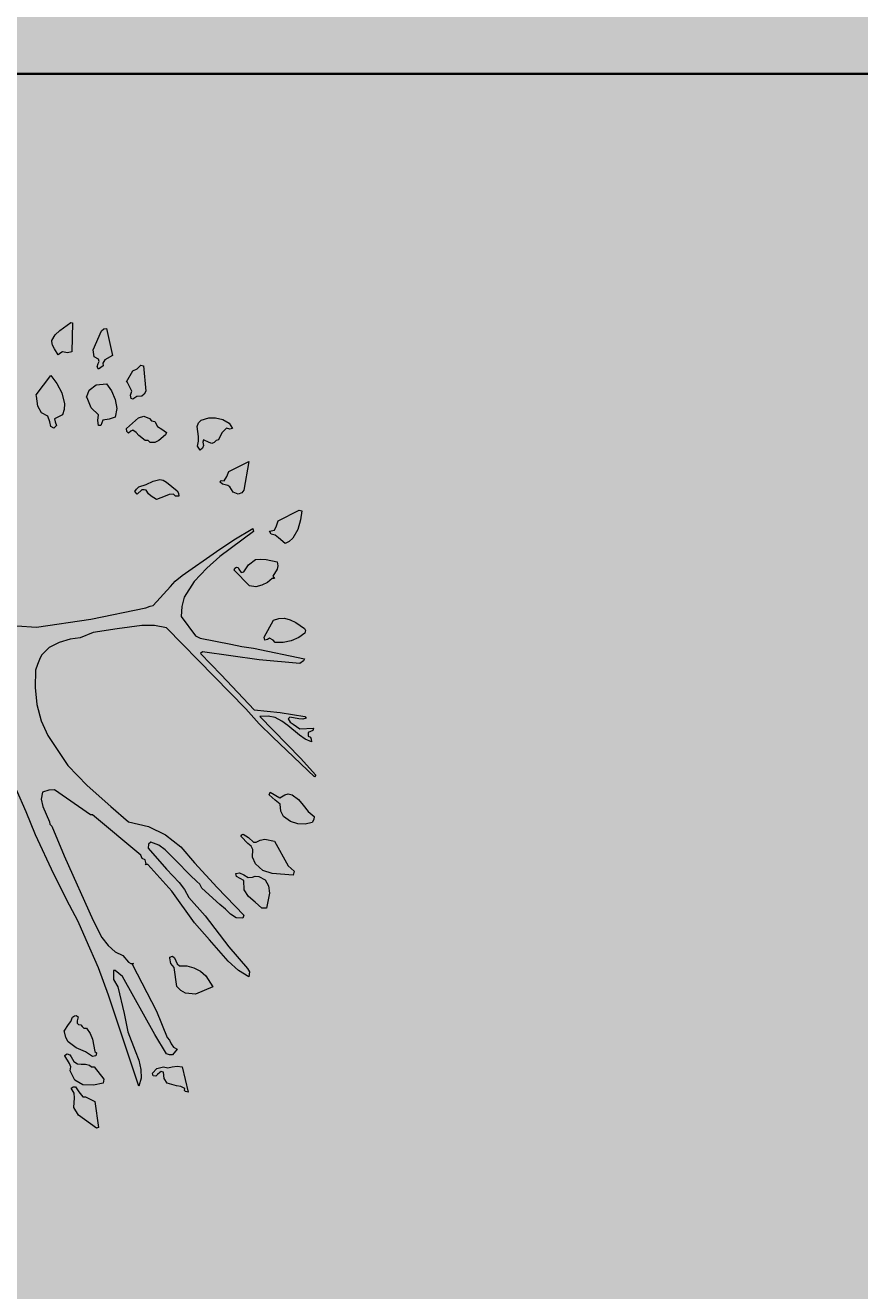
# Model space of a CAD drawing. Units: inches. Extents: x 84 to 1044, y -280 to 906.
# Tile 96 of 105: x 804 to 826, y 479 to 512. Entities that reach past the tile are written whole.
import ezdxf

# ---------------------------------------------------------------- set-up
doc = ezdxf.new("R2010")
doc.units = ezdxf.units.IN
for name, color, linetype, lineweight in [('A-ANNO-DIMS', 2, 'Continuous', 18), ('L-PLNT', 114, 'Continuous', 15), ('WALL', 250, 'Continuous', 35)]:
    doc.layers.add(name, color=color, linetype=linetype, lineweight=lineweight)
doc.layers.add('A-WALL-PATT', color=251, linetype='Continuous', lineweight=9, true_color=0x636466)
doc.layers.add('L-PLNT-PATT', color=9, linetype='Continuous', lineweight=9, true_color=0xafd9aa)
doc.styles.get("Standard").update_dxf_attribs({"font": 'arial.ttf'})
doc.dimstyles.get("Standard").update_dxf_attribs({"dimtxt": 0.18, "dimasz": 0.18, "dimexe": 0.18, "dimexo": 0.0625, "dimgap": 0.09, "dimtad": 0, "dimtih": 1, "dimtoh": 1, "dimdec": 4, "dimzin": 0, "dimdsep": 46, "dimtxsty": 'Standard', "dimcen": 0.09, "dimadec": 0, "dimazin": 0, "dimtfac": 1, "dimtdec": 4, "dimtofl": 0, "dimtmove": 0, "dimatfit": 3, "dimfxl": 1, "dimtolj": 1, "dimtzin": 0, "dimarcsym": 0})

# ---------------------------------------------------------------- blocks, each defined once
blk = doc.blocks.new('A$C37E508DF')
for p, q in [((0.9605, 1.4257), (0.9686, 1.4334)), ((0.9686, 1.4334), (0.9875, 1.4476)), ((0.9875, 1.4476), (0.9905, 1.4467)), ((0.9905, 1.4467), (0.9896, 1.3966)), ((1.0269, 1.3996), (1.0411, 1.433)), ((1.0411, 1.433), (1.045, 1.4365)), ((1.045, 1.4365), (1.0497, 1.4369)), ((1.0497, 1.4369), (1.0604, 1.3901)), ((0.9545, 1.4159), (0.9605, 1.4257)), ((0.9549, 1.4146), (0.9545, 1.4159)), ((0.9558, 1.4077), (0.9549, 1.4146)), ((0.9592, 1.4017), (0.9558, 1.4077)), ((0.966, 1.3914), (0.9592, 1.4017)), ((0.9703, 1.3944), (0.966, 1.3914)), ((0.9733, 1.3966), (0.9703, 1.3944)), ((0.9819, 1.3944), (0.9733, 1.3966)), ((0.9896, 1.3966), (0.9819, 1.3944)), ((1.0282, 1.3876), (1.0269, 1.3996)), ((1.0359, 1.3833), (1.0282, 1.3876)), ((1.0604, 1.3901), (1.0471, 1.3824)), ((1.0334, 1.37), (1.0351, 1.376)), ((1.0359, 1.3661), (1.0334, 1.37)), ((1.0351, 1.376), (1.0368, 1.3794)), ((1.0368, 1.3794), (1.0359, 1.3833)), ((1.0441, 1.3717), (1.0359, 1.3661)), ((1.0471, 1.3824), (1.0432, 1.3764)), ((1.0432, 1.3764), (1.0441, 1.3717)), ((1.0955, 1.3631), (1.1033, 1.367)), ((1.1033, 1.367), (1.1097, 1.373)), ((1.1097, 1.373), (1.114, 1.3717)), ((1.114, 1.3717), (1.1183, 1.328)), ((0.9274, 1.3215), (0.9532, 1.3554)), ((0.9532, 1.3554), (0.9635, 1.3413)), ((1.0848, 1.3443), (1.0955, 1.3631)), ((1.0861, 1.343), (1.0848, 1.3443)), ((0.9279, 1.3194), (0.9274, 1.3215)), ((0.9635, 1.3413), (0.9721, 1.325)), ((0.9721, 1.325), (0.9768, 1.3061)), ((1.0149, 1.3172), (1.0171, 1.3232)), ((1.0171, 1.3232), (1.0197, 1.3297)), ((1.0197, 1.3297), (1.0321, 1.3387)), ((1.0321, 1.3387), (1.0497, 1.3404)), ((1.0497, 1.3404), (1.0587, 1.3284)), ((1.0587, 1.3284), (1.0651, 1.3134)), ((1.0938, 1.328), (1.0861, 1.343)), ((1.0917, 1.3207), (1.0938, 1.328)), ((1.1153, 1.3228), (1.111, 1.3194)), ((1.1183, 1.328), (1.1153, 1.3228)), ((0.9305, 1.3018), (0.9279, 1.3194)), ((0.9365, 1.2902), (0.9305, 1.3018)), ((0.9768, 1.3061), (0.9763, 1.2962)), ((1.0162, 1.3164), (1.0149, 1.3172)), ((1.0231, 1.2988), (1.0162, 1.3164)), ((1.0651, 1.3134), (1.0677, 1.2975)), ((1.0925, 1.3151), (1.0917, 1.3207)), ((1.0955, 1.3138), (1.0925, 1.3151)), ((1.1028, 1.3185), (1.0955, 1.3138)), ((1.111, 1.3194), (1.1028, 1.3185)), ((0.9476, 1.2842), (0.9365, 1.2902)), ((0.951, 1.2748), (0.9476, 1.2842)), ((0.9733, 1.2868), (0.9596, 1.2799)), ((0.9596, 1.2799), (0.9605, 1.2744)), ((0.9763, 1.2962), (0.9733, 1.2868)), ((1.0359, 1.2868), (1.0231, 1.2988)), ((1.0347, 1.2769), (1.0359, 1.2868)), ((1.0432, 1.2774), (1.0402, 1.2679)), ((1.0544, 1.2791), (1.0432, 1.2774)), ((1.0647, 1.2829), (1.0544, 1.2791)), ((1.0677, 1.2975), (1.0647, 1.2829)), ((1.0848, 1.2628), (1.1054, 1.2817)), ((1.1054, 1.2817), (1.1148, 1.2842)), ((1.1148, 1.2842), (1.1247, 1.2804)), ((1.1247, 1.2804), (1.1281, 1.2765)), ((1.21, 1.2726), (1.2147, 1.2774)), ((1.2147, 1.2774), (1.2276, 1.2817)), ((1.2276, 1.2817), (1.2392, 1.2817)), ((1.2392, 1.2817), (1.2521, 1.2787)), ((1.2521, 1.2787), (1.2632, 1.2722)), ((0.9532, 1.2666), (0.951, 1.2748)), ((0.9583, 1.2636), (0.9532, 1.2666)), ((0.9626, 1.2679), (0.9583, 1.2636)), ((0.9605, 1.2744), (0.9626, 1.2679)), ((1.0359, 1.2679), (1.0347, 1.2769)), ((1.0402, 1.2679), (1.0359, 1.2679)), ((1.0852, 1.2576), (1.0848, 1.2628)), ((1.0883, 1.2546), (1.0852, 1.2576)), ((1.0921, 1.2585), (1.0883, 1.2546)), ((1.0955, 1.2602), (1.0921, 1.2585)), ((1.1015, 1.2559), (1.0955, 1.2602)), ((1.1063, 1.2508), (1.1015, 1.2559)), ((1.1281, 1.2765), (1.1341, 1.2752)), ((1.1341, 1.2752), (1.1384, 1.2666)), ((1.1384, 1.2666), (1.1461, 1.2619)), ((1.1461, 1.2619), (1.1539, 1.2559)), ((1.1539, 1.2559), (1.1526, 1.2521)), ((1.2075, 1.2666), (1.21, 1.2726)), ((1.2096, 1.2491), (1.2075, 1.2666)), ((1.2585, 1.2636), (1.2503, 1.2551)), ((1.2645, 1.2615), (1.2585, 1.2636)), ((1.2632, 1.2722), (1.2692, 1.2628)), ((1.2692, 1.2628), (1.2645, 1.2615)), ((1.117, 1.2422), (1.1063, 1.2508)), ((1.1221, 1.2418), (1.117, 1.2422)), ((1.126, 1.2388), (1.1221, 1.2418)), ((1.1337, 1.2388), (1.126, 1.2388)), ((1.141, 1.2422), (1.1337, 1.2388)), ((1.1526, 1.2521), (1.141, 1.2422)), ((1.2079, 1.2323), (1.21, 1.2409)), ((1.21, 1.2409), (1.2096, 1.2491)), ((1.2186, 1.2332), (1.2169, 1.2285)), ((1.2186, 1.2431), (1.2173, 1.2392)), ((1.2173, 1.2392), (1.2186, 1.2332)), ((1.2285, 1.2383), (1.2186, 1.2431)), ((1.2328, 1.2366), (1.2285, 1.2383)), ((1.2371, 1.2388), (1.2328, 1.2366)), ((1.2405, 1.2418), (1.2371, 1.2388)), ((1.2448, 1.2431), (1.2405, 1.2418)), ((1.2503, 1.2551), (1.2448, 1.2431)), ((1.2126, 1.2251), (1.2079, 1.2323)), ((1.2169, 1.2285), (1.2126, 1.2251)), ((1.2628, 1.1882), (1.2975, 1.2053)), ((1.2975, 1.2053), (1.2885, 1.1556)), ((1.1187, 1.1655), (1.1307, 1.1714)), ((1.1307, 1.1714), (1.1423, 1.1744)), ((1.1423, 1.1744), (1.1483, 1.1732)), ((1.1483, 1.1732), (1.1539, 1.1693)), ((1.1539, 1.1693), (1.1727, 1.1543)), ((1.2469, 1.1702), (1.2495, 1.1723)), ((1.2478, 1.1693), (1.2469, 1.1702)), ((1.2516, 1.1659), (1.2478, 1.1693)), ((1.2495, 1.1723), (1.2546, 1.1719)), ((1.2546, 1.1719), (1.2589, 1.1792)), ((1.2589, 1.1792), (1.2628, 1.1882)), ((1.099, 1.153), (1.102, 1.1573)), ((1.1033, 1.1487), (1.099, 1.153)), ((1.102, 1.1573), (1.1063, 1.1612)), ((1.111, 1.156), (1.1033, 1.1487)), ((1.1063, 1.1612), (1.1187, 1.1655)), ((1.1153, 1.1564), (1.111, 1.156)), ((1.1191, 1.1556), (1.1153, 1.1564)), ((1.1226, 1.1492), (1.1191, 1.1556)), ((1.1273, 1.1453), (1.1226, 1.1492)), ((1.1367, 1.1393), (1.1273, 1.1453)), ((1.1517, 1.1453), (1.1367, 1.1393)), ((1.1586, 1.1483), (1.1517, 1.1453)), ((1.1663, 1.1487), (1.1586, 1.1483)), ((1.1697, 1.1449), (1.1663, 1.1487)), ((1.1727, 1.1543), (1.1749, 1.1504)), ((1.1749, 1.1504), (1.1757, 1.1449)), ((1.2563, 1.1646), (1.2516, 1.1659)), ((1.2611, 1.1637), (1.2563, 1.1646)), ((1.2641, 1.1612), (1.2611, 1.1637)), ((1.2701, 1.1522), (1.2641, 1.1612)), ((1.2791, 1.1487), (1.2701, 1.1522)), ((1.2851, 1.1509), (1.2791, 1.1487)), ((1.2885, 1.1556), (1.2851, 1.1509)), ((1.1757, 1.1449), (1.1697, 1.1449)), ((1.3455, 1.0934), (1.3485, 1.102)), ((1.3485, 1.102), (1.385, 1.1209)), ((1.3875, 1.1037), (1.3828, 1.087)), ((1.385, 1.1209), (1.3897, 1.1196)), ((1.3897, 1.1196), (1.3875, 1.1037)), ((1.3057, 1.0835), (1.2469, 1.0402)), ((1.2713, 1.0694), (1.3044, 1.0887)), ((1.3044, 1.0887), (1.3057, 1.0835)), ((1.3335, 1.0844), (1.3421, 1.0861)), ((1.3361, 1.0793), (1.3335, 1.0844)), ((1.3434, 1.0771), (1.3361, 1.0793)), ((1.3421, 1.0861), (1.3455, 1.0934)), ((1.3828, 1.087), (1.3738, 1.072)), ((1.2409, 1.0488), (1.2713, 1.0694)), ((1.349, 1.0728), (1.3434, 1.0771)), ((1.3605, 1.063), (1.349, 1.0728)), ((1.3678, 1.0664), (1.3605, 1.063)), ((1.3738, 1.072), (1.3678, 1.0664)), ((1.1813, 1.0072), (1.2409, 1.0488)), ((1.2469, 1.0402), (1.2246, 1.0201)), ((1.2971, 1.0257), (1.3091, 1.0351)), ((1.3091, 1.0351), (1.3185, 1.0355)), ((1.3185, 1.0355), (1.3275, 1.0347)), ((1.2246, 1.0201), (1.2023, 0.9969)), ((1.2718, 1.0162), (1.2731, 1.0197)), ((1.2984, 0.9892), (1.2718, 1.0162)), ((1.2731, 1.0197), (1.2761, 1.0218)), ((1.2761, 1.0218), (1.2786, 1.0209)), ((1.2786, 1.0209), (1.2799, 1.0184)), ((1.2799, 1.0184), (1.2842, 1.0124)), ((1.2842, 1.0124), (1.2885, 1.0136)), ((1.2885, 1.0136), (1.2971, 1.0257)), ((1.3275, 1.0347), (1.3468, 1.0308)), ((1.3468, 1.018), (1.3391, 1.0059)), ((1.3468, 1.0308), (1.3481, 1.0239)), ((1.3481, 1.0239), (1.3468, 1.018)), ((1.1612, 0.9879), (1.1693, 0.9974)), ((1.1693, 0.9974), (1.1813, 1.0072)), ((1.2023, 0.9969), (1.1852, 0.9691)), ((1.3297, 0.9952), (1.3202, 0.9901)), ((1.3378, 1.0016), (1.3297, 0.9952)), ((1.3421, 1.0016), (1.3378, 1.0016)), ((1.3391, 1.0059), (1.3421, 1.0016)), ((1.1311, 0.9549), (1.1612, 0.9879)), ((1.1852, 0.9691), (1.1809, 0.9532)), ((1.3095, 0.9875), (1.2984, 0.9892)), ((1.3202, 0.9901), (1.3095, 0.9875)), ((1.0227, 0.9309), (1.1183, 0.9506)), ((1.1183, 0.9506), (1.1256, 0.954)), ((1.1256, 0.954), (1.1311, 0.9549)), ((1.1809, 0.9532), (1.1796, 0.936)), ((0.9279, 0.9172), (1.0227, 0.9309)), ((1.1796, 0.936), (1.2049, 0.9022)), ((1.3241, 0.9), (1.3404, 0.9292)), ((1.3404, 0.9292), (1.3494, 0.9322)), ((1.3494, 0.9322), (1.3592, 0.9326)), ((1.3592, 0.9326), (1.3695, 0.93)), ((1.3695, 0.93), (1.3794, 0.9253)), ((1.3794, 0.9253), (1.394, 0.9146)), ((0.8936, 0.9193), (0.9279, 0.9172)), ((1.0269, 0.9077), (1.0042, 0.8987)), ((1.0685, 0.9142), (1.0269, 0.9077)), ((1.1114, 0.9198), (1.0685, 0.9142)), ((1.1333, 0.9202), (1.1114, 0.9198)), ((1.1543, 0.9159), (1.1333, 0.9202)), ((1.2371, 0.8314), (1.1543, 0.9159)), ((1.3948, 0.9065), (1.3846, 0.8992)), ((1.394, 0.9146), (1.3957, 0.9112)), ((1.3957, 0.9112), (1.3948, 0.9065)), ((0.9498, 0.8816), (0.9369, 0.8687)), ((0.9673, 0.8906), (0.9498, 0.8816)), ((0.9866, 0.8962), (0.9673, 0.8906)), ((1.0042, 0.8987), (0.9866, 0.8962)), ((1.2049, 0.9022), (1.2126, 0.8983)), ((1.2126, 0.8983), (1.2662, 0.8876)), ((1.2662, 0.8876), (1.2855, 0.8833)), ((1.2855, 0.8833), (1.3057, 0.8807)), ((1.3254, 0.8944), (1.3241, 0.9)), ((1.3301, 0.8957), (1.3254, 0.8944)), ((1.3335, 0.8983), (1.3301, 0.8957)), ((1.3395, 0.8944), (1.3335, 0.8983)), ((1.3434, 0.8906), (1.3395, 0.8944)), ((1.3571, 0.8906), (1.3434, 0.8906)), ((1.3713, 0.8936), (1.3571, 0.8906)), ((1.3846, 0.8992), (1.3713, 0.8936)), ((0.933, 0.861), (0.9296, 0.852)), ((0.9369, 0.8687), (0.933, 0.861)), ((1.2169, 0.8743), (1.2135, 0.8713)), ((1.2135, 0.8713), (1.2491, 0.834)), ((1.3151, 0.8606), (1.2169, 0.8743)), ((1.3057, 0.8807), (1.394, 0.8623)), ((1.3863, 0.8541), (1.3151, 0.8606)), ((1.394, 0.8623), (1.3927, 0.8584)), ((0.9262, 0.8421), (0.9257, 0.8121)), ((0.9296, 0.852), (0.9262, 0.8421)), ((1.3927, 0.8584), (1.3863, 0.8541)), ((1.2919, 0.7752), (1.2371, 0.8314)), ((1.2491, 0.834), (1.3069, 0.7735)), ((0.9257, 0.8121), (0.9287, 0.7825)), ((0.9287, 0.7825), (0.936, 0.7542)), ((1.3151, 0.7487), (1.2919, 0.7752)), ((1.3069, 0.7735), (1.352, 0.7684)), ((0.936, 0.7542), (0.9476, 0.7285)), ((1.3309, 0.7624), (1.3164, 0.7615)), ((1.3164, 0.7615), (1.3871, 0.6891)), ((1.3434, 0.7598), (1.3309, 0.7624)), ((1.355, 0.7538), (1.3434, 0.7598)), ((1.352, 0.7684), (1.3948, 0.7615)), ((1.3653, 0.7461), (1.355, 0.7538)), ((1.3687, 0.7607), (1.3657, 0.7577)), ((1.3657, 0.7577), (1.3691, 0.7521)), ((1.3841, 0.7577), (1.3687, 0.7607)), ((1.3691, 0.7521), (1.3743, 0.7482)), ((1.3914, 0.7572), (1.3841, 0.7577)), ((1.397, 0.759), (1.3914, 0.7572)), ((1.3948, 0.7615), (1.397, 0.759)), ((0.9476, 0.7285), (0.9828, 0.6762)), ((1.3391, 0.7255), (1.3151, 0.7487)), ((1.3854, 0.7294), (1.3653, 0.7461)), ((1.3743, 0.7482), (1.3863, 0.7405)), ((1.3953, 0.7221), (1.3854, 0.7294)), ((1.3863, 0.7405), (1.4099, 0.7414)), ((1.4086, 0.7375), (1.4004, 0.7337)), ((1.4004, 0.7337), (1.4004, 0.7272)), ((1.4004, 0.7272), (1.4047, 0.7255)), ((1.4099, 0.7414), (1.4086, 0.7375)), ((1.4116, 0.6569), (1.3391, 0.7255)), ((1.4064, 0.7178), (1.3953, 0.7221)), ((1.4047, 0.7255), (1.406, 0.7221)), ((1.406, 0.7221), (1.4064, 0.7178)), ((1.3871, 0.6891), (1.4141, 0.6599)), ((0.9828, 0.6762), (1.0162, 0.6415)), ((1.0162, 0.6415), (1.0574, 0.605)), ((1.4141, 0.6599), (1.4116, 0.6569)), ((0.9103, 0.5956), (0.8932, 0.6342)), ((0.9382, 0.6303), (0.936, 0.6179)), ((0.936, 0.6179), (0.939, 0.605)), ((0.9493, 0.6333), (0.9382, 0.6303)), ((0.9596, 0.6342), (0.9493, 0.6333)), ((1.0218, 0.5904), (0.9596, 0.6342)), ((1.3327, 0.6252), (1.3348, 0.6303)), ((1.343, 0.6162), (1.3327, 0.6252)), ((1.3348, 0.6303), (1.3511, 0.62)), ((1.3511, 0.62), (1.3601, 0.6256)), ((1.3601, 0.6256), (1.3661, 0.6269)), ((1.3661, 0.6269), (1.3725, 0.6252)), ((1.3725, 0.6252), (1.3837, 0.6175)), ((1.3837, 0.6175), (1.3918, 0.6072)), ((0.9262, 0.5557), (0.9103, 0.5956)), ((0.939, 0.605), (0.9506, 0.5784)), ((1.0574, 0.605), (1.0883, 0.5784)), ((1.352, 0.6089), (1.343, 0.6162)), ((1.3533, 0.5969), (1.352, 0.6089)), ((1.358, 0.5874), (1.3533, 0.5969)), ((1.3918, 0.6072), (1.4004, 0.5964)), ((1.4004, 0.5964), (1.4111, 0.5874)), ((0.9506, 0.5784), (0.951, 0.5746)), ((0.951, 0.5746), (0.9545, 0.5711)), ((1.0256, 0.5904), (1.0218, 0.5904)), ((1.1097, 0.5205), (1.0256, 0.5904)), ((1.0883, 0.5784), (1.123, 0.5703)), ((1.37, 0.5789), (1.358, 0.5874)), ((1.3824, 0.575), (1.37, 0.5789)), ((1.3953, 0.5746), (1.3824, 0.575)), ((1.4077, 0.5771), (1.3953, 0.5746)), ((1.4103, 0.5823), (1.4077, 0.5771)), ((1.4111, 0.5874), (1.4103, 0.5823)), ((0.9583, 0.4871), (0.9262, 0.5557)), ((0.9545, 0.5711), (0.9759, 0.5193)), ((1.123, 0.5703), (1.1526, 0.5557)), ((1.1526, 0.5557), (1.1792, 0.5347)), ((1.2842, 0.554), (1.2855, 0.5557)), ((1.2842, 0.5527), (1.2842, 0.554)), ((1.2958, 0.5407), (1.2842, 0.5527)), ((1.2855, 0.5557), (1.2876, 0.557)), ((1.2876, 0.557), (1.2971, 0.551)), ((1.2971, 0.551), (1.3057, 0.5433)), ((1.1226, 0.5394), (1.1221, 0.5325)), ((1.1221, 0.5325), (1.1539, 0.4961)), ((1.1268, 0.5433), (1.1226, 0.5394)), ((1.141, 0.5377), (1.1268, 0.5433)), ((1.1521, 0.5296), (1.141, 0.5377)), ((1.1706, 0.5111), (1.1521, 0.5296)), ((1.1792, 0.5347), (1.2027, 0.5072)), ((1.3014, 0.536), (1.2958, 0.5407)), ((1.3044, 0.53), (1.3014, 0.536)), ((1.3039, 0.5167), (1.3044, 0.53)), ((1.3057, 0.5433), (1.3099, 0.5433)), ((1.3099, 0.5433), (1.3172, 0.5467)), ((1.3172, 0.5467), (1.3254, 0.548)), ((1.3254, 0.548), (1.3421, 0.5446)), ((1.3421, 0.5446), (1.3657, 0.5021)), ((0.9759, 0.5193), (1.0269, 0.4069)), ((1.1118, 0.5145), (1.1097, 0.5205)), ((1.117, 0.5124), (1.1118, 0.5145)), ((1.1191, 0.5055), (1.117, 0.5124)), ((1.1955, 0.4858), (1.1706, 0.5111)), ((1.2027, 0.5072), (1.2426, 0.4644)), ((1.3091, 0.5055), (1.3039, 0.5167)), ((0.9853, 0.4335), (0.9583, 0.4871)), ((1.117, 0.5042), (1.1191, 0.5055)), ((1.1217, 0.5042), (1.117, 0.5042)), ((1.1633, 0.4575), (1.1217, 0.5042)), ((1.1539, 0.4961), (1.1762, 0.4729)), ((1.207, 0.4747), (1.1955, 0.4858)), ((1.2748, 0.4884), (1.2812, 0.4897)), ((1.2761, 0.4832), (1.2748, 0.4884)), ((1.2812, 0.4897), (1.2885, 0.4862)), ((1.2885, 0.4862), (1.2962, 0.4815)), ((1.3215, 0.4935), (1.3091, 0.5055)), ((1.3382, 0.4884), (1.3215, 0.4935)), ((1.3743, 0.4858), (1.3382, 0.4884)), ((1.3657, 0.5021), (1.3764, 0.4927)), ((1.3764, 0.4927), (1.3743, 0.4858)), ((1.1762, 0.4729), (1.1856, 0.4605)), ((1.2122, 0.47), (1.207, 0.4747)), ((1.2156, 0.4627), (1.2122, 0.47)), ((1.2469, 0.4348), (1.2156, 0.4627)), ((1.2426, 0.4644), (1.2885, 0.4159)), ((1.2825, 0.4798), (1.2761, 0.4832)), ((1.2885, 0.4764), (1.2825, 0.4798)), ((1.2894, 0.4601), (1.2885, 0.4764)), ((1.2962, 0.4815), (1.3039, 0.482)), ((1.3039, 0.482), (1.3087, 0.4841)), ((1.3087, 0.4841), (1.3147, 0.4832)), ((1.3147, 0.4832), (1.3258, 0.4777)), ((1.3258, 0.4777), (1.3318, 0.4669)), ((1.3318, 0.4669), (1.3331, 0.4545)), ((1.2027, 0.4026), (1.1633, 0.4575)), ((1.1856, 0.4605), (1.1933, 0.4468)), ((1.1933, 0.4468), (1.2212, 0.4146)), ((1.2967, 0.4485), (1.2894, 0.4601)), ((1.3082, 0.4386), (1.2967, 0.4485)), ((1.3331, 0.4545), (1.3284, 0.4284)), ((1.0003, 0.4052), (0.9853, 0.4335)), ((1.2568, 0.4266), (1.2469, 0.4348)), ((1.2658, 0.4176), (1.2568, 0.4266)), ((1.3198, 0.4284), (1.3082, 0.4386)), ((1.3284, 0.4284), (1.3198, 0.4284)), ((1.0145, 0.373), (1.0003, 0.4052)), ((1.0269, 0.4069), (1.0419, 0.3769)), ((1.2289, 0.373), (1.2027, 0.4026)), ((1.2212, 0.4146), (1.2628, 0.361)), ((1.2752, 0.4116), (1.2658, 0.4176)), ((1.2868, 0.4108), (1.2752, 0.4116)), ((1.2885, 0.4159), (1.2868, 0.4108)), ((1.0419, 0.3769), (1.0527, 0.3632)), ((1.0359, 0.3246), (1.0145, 0.373)), ((1.0527, 0.3632), (1.0647, 0.352)), ((1.2615, 0.3362), (1.2289, 0.373)), ((1.2628, 0.361), (1.2949, 0.3233)), ((1.0647, 0.352), (1.078, 0.346)), ((1.078, 0.346), (1.0883, 0.334)), ((1.0883, 0.334), (1.0921, 0.3319)), ((1.0921, 0.3319), (1.0968, 0.3319)), ((1.0968, 0.3319), (1.0947, 0.3306)), ((1.0947, 0.3306), (1.1367, 0.2491)), ((1.1599, 0.3426), (1.1646, 0.3447)), ((1.1599, 0.3413), (1.1599, 0.3426)), ((1.162, 0.3319), (1.1599, 0.3413)), ((1.1676, 0.325), (1.162, 0.3319)), ((1.1646, 0.3447), (1.168, 0.3417)), ((1.168, 0.3417), (1.1702, 0.3366)), ((1.1702, 0.3366), (1.1727, 0.3314)), ((1.1727, 0.3314), (1.177, 0.3276)), ((1.2795, 0.3199), (1.2615, 0.3362)), ((1.0535, 0.2766), (1.0359, 0.3246)), ((1.0647, 0.3199), (1.0617, 0.3194)), ((1.0617, 0.3194), (1.0617, 0.304)), ((1.0711, 0.3147), (1.0647, 0.3199)), ((1.0775, 0.3092), (1.0711, 0.3147)), ((1.1341, 0.2084), (1.0775, 0.3092)), ((1.1719, 0.292), (1.1676, 0.325)), ((1.177, 0.3276), (1.1895, 0.3276)), ((1.1895, 0.3276), (1.2019, 0.3246)), ((1.2019, 0.3246), (1.2135, 0.3186)), ((1.2135, 0.3186), (1.2225, 0.3104)), ((1.2225, 0.3104), (1.2349, 0.2911)), ((1.2975, 0.3087), (1.2795, 0.3199)), ((1.2949, 0.3233), (1.2988, 0.3173)), ((1.2988, 0.3173), (1.2975, 0.3087)), ((1.0617, 0.304), (1.0698, 0.2911)), ((1.0698, 0.2911), (1.0805, 0.2448)), ((1.1792, 0.2847), (1.1719, 0.292)), ((1.2349, 0.2911), (1.2049, 0.2783)), ((1.0861, 0.1775), (1.0535, 0.2766)), ((1.1873, 0.28), (1.1792, 0.2847)), ((1.2049, 0.2783), (1.1873, 0.28)), ((1.0805, 0.2448), (1.087, 0.2127)), ((1.1367, 0.2491), (1.1556, 0.2032)), ((0.9759, 0.214), (0.9836, 0.226)), ((0.9836, 0.226), (0.9879, 0.2311)), ((0.9879, 0.2311), (0.9905, 0.2384)), ((0.9905, 0.2384), (0.9943, 0.241)), ((0.9943, 0.241), (0.9973, 0.2414)), ((0.9973, 0.2414), (1.0003, 0.2393)), ((1.0003, 0.2393), (0.9986, 0.232)), ((0.9986, 0.232), (0.9986, 0.2281)), ((0.9986, 0.2281), (1.0012, 0.2255)), ((1.0012, 0.2255), (1.0051, 0.2251)), ((1.0051, 0.2251), (1.0076, 0.2225)), ((1.0076, 0.2225), (1.0106, 0.2195)), ((0.9768, 0.2127), (0.9759, 0.214)), ((0.9789, 0.2028), (0.9768, 0.2127)), ((0.9832, 0.1955), (0.9789, 0.2028)), ((1.0106, 0.2195), (1.0149, 0.2191)), ((1.0149, 0.2191), (1.0214, 0.2101)), ((1.0214, 0.2101), (1.0252, 0.2002)), ((1.0252, 0.2002), (1.0295, 0.1788)), ((1.087, 0.2127), (1.0998, 0.1797)), ((1.1543, 0.1749), (1.1341, 0.2084)), ((1.1556, 0.2032), (1.1594, 0.1985)), ((1.1594, 0.1985), (1.1624, 0.1921)), ((0.9969, 0.1852), (0.9832, 0.1955)), ((1.0132, 0.1779), (0.9969, 0.1852)), ((1.0256, 0.1698), (1.0132, 0.1779)), ((1.0295, 0.1788), (1.0325, 0.1762)), ((1.0325, 0.1762), (1.0312, 0.1711)), ((1.1063, 0.1183), (1.0861, 0.1775)), ((1.0998, 0.1797), (1.1058, 0.1634)), ((1.1624, 0.1921), (1.1663, 0.1861)), ((1.1727, 0.1827), (1.1646, 0.1732)), ((1.1663, 0.1861), (1.1727, 0.1827)), ((0.9768, 0.1719), (0.9811, 0.1749)), ((0.9776, 0.1711), (0.9768, 0.1719)), ((0.9853, 0.1578), (0.9776, 0.1711)), ((0.9811, 0.1749), (0.9858, 0.1728)), ((0.9879, 0.1518), (0.9853, 0.1578)), ((0.9858, 0.1728), (0.9884, 0.1694)), ((0.9884, 0.1694), (0.9931, 0.1616)), ((0.9931, 0.1616), (0.9991, 0.1574)), ((0.9991, 0.1574), (1.0059, 0.1565)), ((1.0059, 0.1565), (1.0132, 0.1565)), ((1.0132, 0.1565), (1.0205, 0.1548)), ((1.0205, 0.1548), (1.0235, 0.1522)), ((1.0312, 0.1711), (1.0256, 0.1698)), ((1.1058, 0.1634), (1.1097, 0.1475)), ((1.1594, 0.1728), (1.1543, 0.1749)), ((1.1646, 0.1732), (1.1594, 0.1728)), ((0.9866, 0.1453), (0.9879, 0.1518)), ((0.9948, 0.1291), (0.9866, 0.1453)), ((1.0235, 0.1522), (1.0282, 0.1518)), ((1.0282, 0.1518), (1.0454, 0.1303)), ((1.1101, 0.1325), (1.1063, 0.1183)), ((1.1097, 0.1475), (1.1101, 0.1325)), ((1.1298, 0.1411), (1.1376, 0.1492)), ((1.1311, 0.1364), (1.1298, 0.1411)), ((1.1354, 0.1359), (1.1311, 0.1364)), ((1.1384, 0.1389), (1.1354, 0.1359)), ((1.1376, 0.1492), (1.1491, 0.1518)), ((1.1423, 0.1423), (1.1384, 0.1389)), ((1.1449, 0.1441), (1.1423, 0.1423)), ((1.1491, 0.1428), (1.1449, 0.1441)), ((1.1491, 0.1518), (1.1564, 0.1505)), ((1.1504, 0.132), (1.1491, 0.1428)), ((1.1564, 0.1505), (1.1642, 0.1518)), ((1.1642, 0.1518), (1.1727, 0.1531)), ((1.1727, 0.1531), (1.1813, 0.1518)), ((1.1813, 0.1518), (1.192, 0.108)), ((0.9884, 0.1149), (0.9918, 0.117)), ((0.9935, 0.1063), (0.9884, 0.1149)), ((0.9918, 0.117), (0.9961, 0.1175)), ((1.0089, 0.1205), (0.9948, 0.1291)), ((0.9961, 0.1175), (1.0016, 0.1085)), ((1.0274, 0.12), (1.0089, 0.1205)), ((1.0441, 0.1239), (1.0274, 0.12)), ((1.0454, 0.1303), (1.0441, 0.1239)), ((1.1556, 0.1239), (1.1504, 0.132)), ((1.1714, 0.1192), (1.1556, 0.1239)), ((1.1792, 0.1179), (1.1714, 0.1192)), ((1.186, 0.1145), (1.1792, 0.1179)), ((1.1856, 0.111), (1.186, 0.1145)), ((1.1873, 0.1093), (1.1856, 0.111)), ((0.9931, 0.081), (0.9943, 0.0982)), ((0.9943, 0.0982), (0.9935, 0.1063)), ((1.0016, 0.1085), (1.0089, 0.0999)), ((1.0089, 0.0999), (1.0132, 0.0999)), ((1.0132, 0.0999), (1.0295, 0.0917)), ((1.0295, 0.0917), (1.0359, 0.0463)), ((1.192, 0.108), (1.1873, 0.1093)), ((1.0012, 0.0677), (0.9931, 0.081)), ((1.0325, 0.0454), (1.0012, 0.0677)), ((1.0359, 0.0463), (1.0325, 0.0454))]:
    blk.add_line(p, q)
blk = doc.blocks.new('*D62')
at = {"layer": 'A-ANNO-DIMS', "color": 0, "lineweight": -2, "transparency": 16777216}
for p, q in [((203.179, 709.183), (203.179, 905.9)), ((896.074, 400.183), (896.074, 905.9)), ((203.359, 905.72), (549.232, 905.72)), ((895.894, 905.72), (550.021, 905.72))]:
    blk.add_line(p, q, dxfattribs=at)
at = {"layer": 'A-ANNO-DIMS', "color": 0, "transparency": 16777216}
for points in [[(203.359, 905.75), (203.359, 905.69), (203.179, 905.72)], [(895.894, 905.75), (895.894, 905.69), (896.074, 905.72)]]:
    blk.add_solid(points, dxfattribs=at)
at = {"layer": 'Defpoints', "color": 0, "transparency": 16777216}
for p in [(896.074, 905.72), (203.179, 709.12), (896.074, 400.12)]:
    blk.add_point(p, dxfattribs=at)
at = {"layer": 'A-ANNO-DIMS', "color": 0, "transparency": 16777216, "insert": (549.627, 905.72), "char_height": 0.18, "attachment_point": 5}
blk.add_mtext('\\A1;692.9', dxfattribs=at)

msp = doc.modelspace()

# ---------------------------------------------------------------- hatches: boundary and pattern name
at = {"layer": 'A-WALL-PATT', "transparency": 33554597}
h = msp.add_hatch(color=256, dxfattribs=at)
h.dxf.hatch_style = 1
h.paths.add_polyline_path([(671.074, 100.12), (647.074, 100.12), (647.074, 160.12), (641.074, 160.12), (620.824, 160.12), (620.824, 151.12), (638.074, 151.12), (638.074, 91.12), (671.074, 91.12)])
h.paths.add_polyline_path([(791.074, 100.12), (743.074, 100.12), (743.074, 91.12), (791.074, 91.12)])
h.paths.add_polyline_path([(896.074, 346.12), (887.074, 346.12), (887.074, 334.12), (870.955, 334.12), (833.074, 334.12), (804.574, 334.12), (804.574, 328.12), (887.074, 328.12), (887.074, 100.12), (863.074, 100.12), (863.074, 91.12), (896.074, 91.12)])
h.paths.add_polyline_path([(507.574, 154.729), (507.574, 160.12), (464.074, 160.12), (464.074, 247.12), (641.074, 247.12), (641.074, 208.12), (647.074, 208.12), (647.074, 328.12), (659.074, 328.12), (659.074, 334.12), (617.074, 334.12), (617.074, 328.12), (641.074, 328.12), (641.074, 256.12), (545.074, 256.12), (545.074, 328.12), (569.074, 328.12), (569.074, 334.12), (518.074, 334.12), (518.074, 325.12), (536.074, 325.12), (536.074, 256.12), (464.074, 256.12), (464.074, 325.12), (482.074, 325.12), (482.074, 334.12), (455.074, 334.12), (455.074, 160.12), (413.127, 160.12), (413.127, 151.12), (455.074, 151.12), (455.074, 91.12), (464.074, 91.12), (464.074, 151.12), (507.574, 151.12)])
h.paths.add_polyline_path([(572.824, 160.12), (555.574, 160.12), (555.574, 151.12), (572.824, 151.12)], flags=17)
h.paths.add_polyline_path([(341.127, 160.12), (299.179, 160.12), (299.179, 211.12), (294.179, 211.12), (290.179, 211.12), (290.179, 151.12), (341.127, 151.12)])
h.paths.add_polyline_path([(299.179, 256.12), (212.179, 256.12), (212.179, 274.12), (203.179, 274.12), (203.179, 247.12), (299.179, 247.12)])
h.paths.add_polyline_path([(212.179, 514.12), (398.074, 514.12), (398.074, 519.12), (398.074, 520.12), (212.179, 520.12), (212.179, 574.12), (203.179, 574.12), (203.179, 310.12), (212.179, 310.12), (212.179, 328.12), (290.179, 328.12), (290.179, 292.12), (299.179, 292.12), (299.179, 328.12), (332.179, 328.12), (332.179, 334.12), (212.179, 334.12)])
h.paths.add_polyline_path([(287.127, 709.12), (203.179, 709.12), (203.179, 646.12), (212.179, 646.12), (212.179, 700.12), (287.127, 700.12)])
h.paths.add_polyline_path([(470.074, 709.12), (359.127, 709.12), (359.127, 700.12), (434.074, 700.12), (434.074, 574.12), (440.074, 574.12), (440.074, 622.12), (464.074, 622.12), (464.074, 628.12), (440.074, 628.12), (440.074, 700.12), (470.074, 700.12)])
h.paths.add_polyline_path([(572.074, 709.12), (506.074, 709.12), (506.074, 700.12), (536.074, 700.12), (536.074, 628.12), (494.074, 628.12), (494.074, 622.12), (536.074, 622.12), (536.074, 520.12), (440.074, 520.12), (440.074, 544.12), (434.074, 544.12), (434.074, 514.12), (644.074, 514.12), (644.074, 519.12), (644.074, 544.12), (638.074, 544.12), (638.074, 520.12), (542.074, 520.12), (542.074, 622.12), (584.074, 622.12), (584.074, 628.12), (542.074, 628.12), (542.074, 700.12), (572.074, 700.12)])
h.paths.add_polyline_path([(698.074, 709.12), (608.074, 709.12), (608.074, 700.12), (638.074, 700.12), (638.074, 628.12), (614.074, 628.12), (614.074, 622.12), (638.074, 622.12), (638.074, 574.12), (644.074, 574.12), (644.074, 700.12), (698.074, 700.12)])
h.paths.add_polyline_path([(833.074, 709.12), (770.074, 709.12), (770.074, 700.12), (824.074, 700.12), (824.074, 646.12), (833.074, 646.12)])
h.paths.add_polyline_path([(833.074, 574.12), (824.074, 574.12), (824.074, 520.12), (791.244, 520.12), (712.904, 520.12), (680.074, 520.12), (680.074, 514.12), (695.074, 514.12), (695.074, 491.62), (704.074, 491.62), (704.074, 511.12), (833.074, 511.12)])
h.paths.add_polyline_path([(704.074, 419.62), (695.074, 419.62), (695.074, 370.12), (704.074, 370.12)])
h.paths.add_polyline_path([(896.074, 400.12), (833.074, 400.12), (833.074, 364.12), (839.074, 364.12), (839.074, 394.12), (887.074, 394.12), (887.074, 382.12), (896.074, 382.12)])
h.paths.add_polyline_path([(732.574, 334.12), (695.074, 334.12), (695.074, 328.12), (732.574, 328.12)])
at = {"layer": 'L-PLNT-PATT', "transparency": 33554597}
h = msp.add_hatch(color=256, dxfattribs=at)
h.dxf.hatch_style = 1
h.paths.add_polyline_path([(896.074, 511.12), (704.074, 511.12), (704.074, 491.62), (704.074, 419.62), (704.074, 400.12), (833.074, 400.12), (896.074, 400.12)])

# ---------------------------------------------------------------- linework, layer by layer
at = {"layer": 'WALL'}
msp.add_line((896.074, 511.12), (704.074, 511.12), dxfattribs=at)

# ---------------------------------------------------------------- block references
at = {"layer": 'L-PLNT', "xscale": 15.19586232982809, "yscale": 15.19586232982809, "zscale": 15.19586232982809}
msp.add_blockref('A$C37E508DF', (789.857, 482.553), dxfattribs=at)

# ---------------------------------------------------------------- dimensions: what is measured, and where the dimension line sits
at = {"layer": 'A-ANNO-DIMS'}
dim = msp.add_linear_dim(base=(896.074, 905.72), p1=(203.179, 709.12), p2=(896.074, 400.12), dimstyle='Standard', override={"dimdec": 1, "dimlfac": 1, "dimrnd": 0, "dimzin": 0, "dimdsep": 46, "dimlunit": 2}, dxfattribs=at)
dim.commit()
dim.dimension.update_dxf_attribs({"geometry": '*D62', "text_midpoint": (549.627, 905.72)})

doc.saveas('drawing.dxf')
